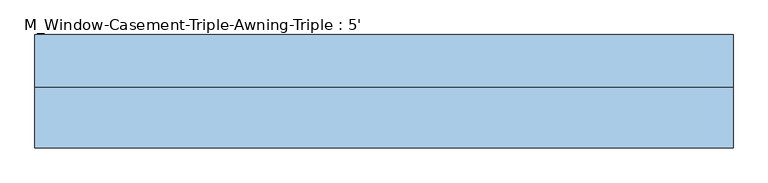
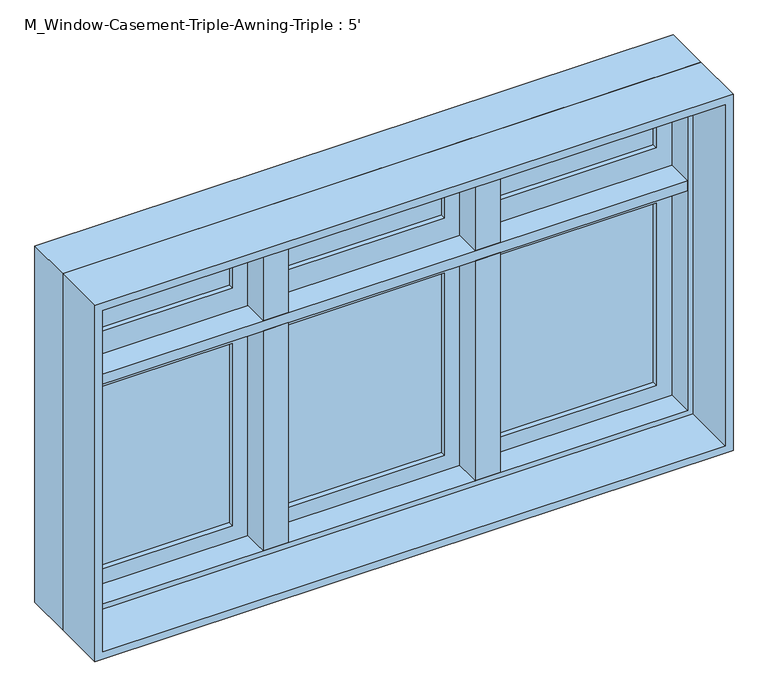
"""IFC4 building model written with IfcOpenShell, lengths in millimetres: window geometry, M_Window-Casement-Triple-Awning-Triple : 5'."""

from ifc_helpers import new_model, si_unit, frame, origin, place, context, project, spatial, polyline, outline, extrude, faceted_brep, source, transform, mapped, element, save


def m_window_casement_triple_awning_triple_5_96d5a87e(model_context):
    return source(origin(), model_context, "Body", "SolidModel", [
        faceted_brep([(730.25, 82.55, 1768.25), (730.25, 19.05, 1768.25), (-730.25, 19.05, 1768.25), (-730.25, 82.55, 1768.25), (749.3, 133.35, 1787.3), (749.3, 82.55, 1787.3), (-749.3, 82.55, 1787.3), (-749.3, 133.35, 1787.3), (762.0, 19.05, 1800.0), (762.0, 133.35, 1800.0), (-762.0, 133.35, 1800.0), (-762.0, 19.05, 1800.0), (-730.25, 19.05, 931.75), (-730.25, 82.55, 931.75), (-749.3, 82.55, 912.7), (-749.3, 133.35, 912.7), (-762.0, 133.35, 900.0), (-762.0, 19.05, 900.0), (730.25, 19.05, 931.75), (730.25, 82.55, 931.75), (749.3, 82.55, 912.7), (749.3, 133.35, 912.7), (762.0, 133.35, 900.0), (762.0, 19.05, 900.0)], [[[0, 1, 2, 3]], [[4, 5, 6, 7]], [[8, 9, 10, 11]], [[3, 2, 12, 13]], [[7, 6, 14, 15]], [[11, 10, 16, 17]], [[13, 12, 18, 19]], [[15, 14, 20, 21]], [[17, 16, 22, 23]], [[11, 17, 23, 8], [1, 18, 12, 2]], [[19, 18, 1, 0]], [[5, 20, 14, 6], [3, 13, 19, 0]], [[21, 20, 5, 4]], [[23, 22, 9, 8]], [[9, 22, 16, 10], [7, 15, 21, 4]]]),
        extrude(outline(polyline([(1800.0, -762.0), (900.0, -762.0), (900.0, 762.0), (1800.0, 762.0), (1800.0, -762.0)]), holes=[polyline([(1780.95, 742.95), (919.05, 742.95), (919.05, -742.95), (1780.95, -742.95), (1780.95, 742.95)])]), frame((0.0, -114.3, 0.0), z_axis=(0.0, 1.0, 0.0), x_axis=(0.0, 0.0, 1.0)), (0.0, 0.0, 1.0), 133.35),
        extrude(outline(polyline([(912.7, 749.3), (1487.3, 749.3), (1487.3, 262.4666667), (912.7, 262.4666667), (912.7, 749.3)]), holes=[polyline([(969.85, 319.6166667), (1430.15, 319.6166667), (1430.15, 692.15), (969.85, 692.15), (969.85, 319.6166667)])]), frame((0.0, 82.55, 0.0), z_axis=(0.0, 1.0, 0.0), x_axis=(0.0, 0.0, 1.0)), (0.0, 0.0, 1.0), 44.45),
        extrude(outline(polyline([(692.15, 114.3), (692.15, 107.95), (319.6166667, 107.95), (319.6166667, 114.3), (692.15, 114.3)])), frame((0.0, 0.0, 969.85), z_axis=(0.0, 0.0, 1.0), x_axis=(1.0, 0.0, 0.0)), (0.0, 0.0, 1.0), 460.3),
        extrude(outline(polyline([(319.6166667, 95.25), (319.6166667, 101.6), (692.15, 101.6), (692.15, 95.25), (319.6166667, 95.25)])), frame((0.0, 0.0, 969.85), z_axis=(0.0, 0.0, 1.0), x_axis=(1.0, 0.0, 0.0)), (0.0, 0.0, 1.0), 460.3),
        extrude(outline(polyline([(-319.6166667, 114.3), (-319.6166667, 107.95), (-692.15, 107.95), (-692.15, 114.3), (-319.6166667, 114.3)])), frame((0.0, 0.0, 969.85), z_axis=(0.0, 0.0, 1.0), x_axis=(1.0, 0.0, 0.0)), (0.0, 0.0, 1.0), 460.3),
        extrude(outline(polyline([(-692.15, 95.25), (-692.15, 101.6), (-319.6166667, 101.6), (-319.6166667, 95.25), (-692.15, 95.25)])), frame((0.0, 0.0, 969.85), z_axis=(0.0, 0.0, 1.0), x_axis=(1.0, 0.0, 0.0)), (0.0, 0.0, 1.0), 460.3),
        extrude(outline(polyline([(186.2666667, 114.3), (186.2666667, 107.95), (-186.2666667, 107.95), (-186.2666667, 114.3), (186.2666667, 114.3)])), frame((0.0, 0.0, 969.85), z_axis=(0.0, 0.0, 1.0), x_axis=(1.0, 0.0, 0.0)), (0.0, 0.0, 1.0), 460.3),
        extrude(outline(polyline([(-186.2666667, 95.25), (-186.2666667, 101.6), (186.2666667, 101.6), (186.2666667, 95.25), (-186.2666667, 95.25)])), frame((0.0, 0.0, 969.85), z_axis=(0.0, 0.0, 1.0), x_axis=(1.0, 0.0, 0.0)), (0.0, 0.0, 1.0), 460.3),
        faceted_brep([(-262.4666667, 82.55, 1487.3), (-282.9768005, 82.55, 1487.3), (-282.9768005, 19.05, 1487.3), (-222.9065328, 19.05, 1487.3), (-222.9065328, 82.55, 1487.3), (-243.4166667, 82.55, 1487.3), (-243.4166667, 133.35, 1487.3), (-262.4666667, 133.35, 1487.3), (-262.4666667, 133.35, 912.7), (-243.4166667, 133.35, 912.7), (-243.4166667, 95.25, 912.7), (-262.4666667, 95.25, 912.7), (-282.9768005, 82.55, 931.75), (-282.9768005, 19.05, 931.75), (-222.9065328, 19.05, 931.75), (-222.9065328, 82.55, 931.75), (-243.4166667, 82.55, 931.75), (-243.4166667, 95.25, 931.75), (-262.4666667, 95.25, 931.75), (-262.4666667, 82.55, 931.75)], [[[0, 1, 2, 3, 4, 5, 6, 7]], [[8, 9, 10, 11]], [[2, 1, 12, 13]], [[3, 2, 13, 14]], [[4, 3, 14, 15]], [[6, 5, 16, 17, 10, 9]], [[0, 7, 8, 11, 18, 19]], [[17, 18, 11, 10]], [[18, 17, 16, 15, 14, 13, 12, 19]], [[1, 0, 19, 12]], [[5, 4, 15, 16]], [[7, 6, 9, 8]]]),
        faceted_brep([(243.4166667, 82.55, 1487.3), (222.9065328, 82.55, 1487.3), (222.9065328, 19.05, 1487.3), (282.9768005, 19.05, 1487.3), (282.9768005, 82.55, 1487.3), (262.4666667, 82.55, 1487.3), (262.4666667, 133.35, 1487.3), (243.4166667, 133.35, 1487.3), (243.4166667, 133.35, 912.7), (262.4666667, 133.35, 912.7), (262.4666667, 95.25, 912.7), (243.4166667, 95.25, 912.7), (222.9065328, 82.55, 931.75), (222.9065328, 19.05, 931.75), (282.9768005, 19.05, 931.75), (282.9768005, 82.55, 931.75), (262.4666667, 82.55, 931.75), (262.4666667, 95.25, 931.75), (243.4166667, 95.25, 931.75), (243.4166667, 82.55, 931.75)], [[[0, 1, 2, 3, 4, 5, 6, 7]], [[8, 9, 10, 11]], [[2, 1, 12, 13]], [[3, 2, 13, 14]], [[4, 3, 14, 15]], [[6, 5, 16, 17, 10, 9]], [[0, 7, 8, 11, 18, 19]], [[17, 18, 11, 10]], [[18, 17, 16, 15, 14, 13, 12, 19]], [[1, 0, 19, 12]], [[5, 4, 15, 16]], [[7, 6, 9, 8]]]),
        extrude(outline(polyline([(-730.25, 19.05), (-730.25, 82.55), (-749.3, 82.55), (-749.3, 133.35), (749.3, 133.35), (749.3, 82.55), (730.25, 82.55), (730.25, 19.05), (-730.25, 19.05)])), frame((0.0, 0.0, 1487.3), z_axis=(0.0, 0.0, 1.0), x_axis=(1.0, 0.0, 0.0)), (0.0, 0.0, 1.0), 25.4),
        extrude(outline(polyline([(692.15, 114.3), (692.15, 107.95), (319.6166667, 107.95), (319.6166667, 114.3), (692.15, 114.3)])), frame((0.0, 0.0, 1569.85), z_axis=(0.0, 0.0, 1.0), x_axis=(1.0, 0.0, 0.0)), (0.0, 0.0, 1.0), 160.3),
        extrude(outline(polyline([(319.6166667, 101.6), (692.15, 101.6), (692.15, 95.25), (319.6166667, 95.25), (319.6166667, 101.6)])), frame((0.0, 0.0, 1569.85), z_axis=(0.0, 0.0, 1.0), x_axis=(1.0, 0.0, 0.0)), (0.0, 0.0, 1.0), 160.3),
        faceted_brep([(-243.4166667, 82.55, 1787.3), (-243.4166667, 133.35, 1787.3), (-262.4666667, 133.35, 1787.3), (-262.4666667, 82.55, 1787.3), (-262.4666667, 82.55, 1512.7), (-262.4666667, 133.35, 1512.7), (-243.4166667, 133.35, 1512.7), (-243.4166667, 82.55, 1512.7), (-222.9065328, 82.55, 1512.7), (-222.9065328, 19.05, 1512.7), (-282.9768005, 19.05, 1512.7), (-282.9768005, 82.55, 1512.7), (-282.9768005, 82.55, 1768.25), (-262.4666667, 82.55, 1768.25), (-282.9768005, 19.05, 1768.25), (-222.9065328, 19.05, 1768.25), (-222.9065328, 82.55, 1768.25), (-243.4166667, 82.55, 1768.25)], [[[0, 1, 2, 3]], [[4, 5, 6, 7, 8, 9, 10, 11]], [[4, 11, 12, 13]], [[11, 10, 14, 12]], [[10, 9, 15, 14]], [[9, 8, 16, 15]], [[8, 7, 17, 16]], [[1, 0, 17, 7, 6]], [[2, 1, 6, 5]], [[3, 2, 5, 4, 13]], [[17, 13, 12, 14, 15, 16]], [[13, 17, 0, 3]]]),
        faceted_brep([(262.4666667, 82.55, 1787.3), (262.4666667, 133.35, 1787.3), (243.4166667, 133.35, 1787.3), (243.4166667, 82.55, 1787.3), (243.4166667, 82.55, 1512.7), (243.4166667, 133.35, 1512.7), (262.4666667, 133.35, 1512.7), (262.4666667, 82.55, 1512.7), (282.9768005, 82.55, 1512.7), (282.9768005, 19.05, 1512.7), (222.9065328, 19.05, 1512.7), (222.9065328, 82.55, 1512.7), (222.9065328, 82.55, 1768.25), (243.4166667, 82.55, 1768.25), (222.9065328, 19.05, 1768.25), (282.9768005, 19.05, 1768.25), (282.9768005, 82.55, 1768.25), (262.4666667, 82.55, 1768.25)], [[[0, 1, 2, 3]], [[4, 5, 6, 7, 8, 9, 10, 11]], [[4, 11, 12, 13]], [[11, 10, 14, 12]], [[10, 9, 15, 14]], [[9, 8, 16, 15]], [[8, 7, 17, 16]], [[1, 0, 17, 7, 6]], [[2, 1, 6, 5]], [[3, 2, 5, 4, 13]], [[17, 13, 12, 14, 15, 16]], [[13, 17, 0, 3]]]),
        extrude(outline(polyline([(1512.7, 749.3), (1787.3, 749.3), (1787.3, 262.4666667), (1512.7, 262.4666667), (1512.7, 749.3)]), holes=[polyline([(1569.85, 319.6166667), (1730.15, 319.6166667), (1730.15, 692.15), (1569.85, 692.15), (1569.85, 319.6166667)])]), frame((0.0, 82.55, 0.0), z_axis=(0.0, 1.0, 0.0), x_axis=(0.0, 0.0, 1.0)), (0.0, 0.0, 1.0), 44.45),
        extrude(outline(polyline([(186.2666667, 114.3), (186.2666667, 107.95), (-186.2666667, 107.95), (-186.2666667, 114.3), (186.2666667, 114.3)])), frame((0.0, 0.0, 1569.85), z_axis=(0.0, 0.0, 1.0), x_axis=(1.0, 0.0, 0.0)), (0.0, 0.0, 1.0), 160.3),
        extrude(outline(polyline([(-186.2666667, 101.6), (186.2666667, 101.6), (186.2666667, 95.25), (-186.2666667, 95.25), (-186.2666667, 101.6)])), frame((0.0, 0.0, 1569.85), z_axis=(0.0, 0.0, 1.0), x_axis=(1.0, 0.0, 0.0)), (0.0, 0.0, 1.0), 160.3),
        extrude(outline(polyline([(-319.6166667, 114.3), (-319.6166667, 107.95), (-692.15, 107.95), (-692.15, 114.3), (-319.6166667, 114.3)])), frame((0.0, 0.0, 1569.85), z_axis=(0.0, 0.0, 1.0), x_axis=(1.0, 0.0, 0.0)), (0.0, 0.0, 1.0), 160.3),
        extrude(outline(polyline([(-692.15, 101.6), (-319.6166667, 101.6), (-319.6166667, 95.25), (-692.15, 95.25), (-692.15, 101.6)])), frame((0.0, 0.0, 1569.85), z_axis=(0.0, 0.0, 1.0), x_axis=(1.0, 0.0, 0.0)), (0.0, 0.0, 1.0), 160.3),
        extrude(outline(polyline([(1487.3, -243.4166667), (912.7, -243.4166667), (912.7, 243.4166667), (1487.3, 243.4166667), (1487.3, -243.4166667)]), holes=[polyline([(1430.15, 186.2666667), (969.85, 186.2666667), (969.85, -186.2666667), (1430.15, -186.2666667), (1430.15, 186.2666667)])]), frame((0.0, 82.55, 0.0), z_axis=(0.0, 1.0, 0.0), x_axis=(0.0, 0.0, 1.0)), (0.0, 0.0, 1.0), 44.45),
        extrude(outline(polyline([(1512.7, 243.4166667), (1787.3, 243.4166667), (1787.3, -243.4166667), (1512.7, -243.4166667), (1512.7, 243.4166667)]), holes=[polyline([(1569.85, -186.2666667), (1730.15, -186.2666667), (1730.15, 186.2666667), (1569.85, 186.2666667), (1569.85, -186.2666667)])]), frame((0.0, 82.55, 0.0), z_axis=(0.0, 1.0, 0.0), x_axis=(0.0, 0.0, 1.0)), (0.0, 0.0, 1.0), 44.45),
        extrude(outline(polyline([(1487.3, -749.3), (912.7, -749.3), (912.7, -262.4666667), (1487.3, -262.4666667), (1487.3, -749.3)]), holes=[polyline([(1430.15, -319.6166667), (969.85, -319.6166667), (969.85, -692.15), (1430.15, -692.15), (1430.15, -319.6166667)])]), frame((0.0, 82.55, 0.0), z_axis=(0.0, 1.0, 0.0), x_axis=(0.0, 0.0, 1.0)), (0.0, 0.0, 1.0), 44.45),
        extrude(outline(polyline([(1512.7, -262.4666667), (1787.3, -262.4666667), (1787.3, -749.3), (1512.7, -749.3), (1512.7, -262.4666667)]), holes=[polyline([(1569.85, -692.15), (1730.15, -692.15), (1730.15, -319.6166667), (1569.85, -319.6166667), (1569.85, -692.15)])]), frame((0.0, 82.55, 0.0), z_axis=(0.0, 1.0, 0.0), x_axis=(0.0, 0.0, 1.0)), (0.0, 0.0, 1.0), 44.45),
    ])


if __name__ == "__main__":
    model = new_model("IFC4")
    model_context = context("Model", 3, world=origin())
    ifc_project = project(units=[si_unit("LENGTHUNIT", "METRE", prefix="MILLI")], contexts=[model_context])
    site = spatial("IfcSite", under=ifc_project)
    building = spatial("IfcBuilding", under=site)
    placement = place(None, origin())
    m_window_casement_triple_awning_triple_5_shape = m_window_casement_triple_awning_triple_5_96d5a87e(model_context)
    element("IfcWindow", 1, ObjectType="M_Window-Casement-Triple-Awning-Triple : 5'", at=placement, inside=building, context=model_context, shape_type="MappedRepresentation", body=[
        mapped(m_window_casement_triple_awning_triple_5_shape, transform((0.0, 0.0, 0.0), x_axis=(1.0, 0.0, 0.0), y_axis=(0.0, 1.0, 0.0), z_axis=(0.0, 0.0, 1.0))),
    ])
    save(model, "model.ifc")

# Revit data of these elements
# Type "M_Window-Casement-Triple-Awning-Triple : 5'"
#   Type Mark = "19"
#   Fire Rating = "0.5h"
#   Assembly Code = "B2020100"
#   Analytic Construction = "Double glazing - domestic"
#   Window Inset [instance default] = 0' - 0"
#   Wall Thickness [instance default] = 0' - 5.90551"
#   One Third Width = 1' - 8"
#   Visual Light Transmittance = 0.81
#   Transom Height = 0' - 11.81102"
#   Thermal Resistance (R) = 1.8146 (h·ft²·°F)/BTU
#   Solar Heat Gain Coefficient = 0.76
#   Sash Width = 1' - 7.16667"
#   Rough Width = 5' - 0.59055"
#   Rough Height = 3' - 0.02362"
#   Open Window Height = 1' - 11.62205"
#   Frame Extension [instance default] = 0' - 0 1/4"
#   Interior Wall Closure [instance default] = 0' - 2.15551"
#   Height = 2' - 11.43307"
#   Heat Transfer Coefficient (U) = 0.5511 BTU/(h·ft²·°F)
#   Exterior Wall Closure [instance default] = 0' - 1 1/4"
#   Extension Jamb [instance default] = 0' - 2.15551"
#   Default Sill Height = 2' - 11.43307"
#   Width = 5' - 0"
#   Top Side Muntin Visibility = yes
#   Top Middle Muntin Visibility = yes
#   Bottom Side Muntin Visibility = yes
#   Bottom Middle Muntin Visibility = yes
#   Interior Trim Visibility [instance default] = yes
#   Exterior Trim Visibility [instance default] = yes
#   Extension Jamb Visibility [instance default] = yes
#   Muntin Pattern = M_Muntin Pattern_2x2 : M_Muntin Pattern_2x2
#   Interior Trim Material = Wood - Stained
#   Interior Trim = M_Trim-Window-Interior-Flat : Picture Frame
#   Interior Frame Material = Wood - Stained
#   Glass Panel Material = Glass
#   Exterior Trim Material = Clad - White
#   Exterior Trim = M_Trim-Window-Exterior-Flat : with Sill
#   Exterior Frame Material = Clad - White
#   Wall Closure = (empty or 0)
# Element 1 (IfcWindow, "M_Window-Casement-Triple-Awning-Triple : 5'")
#   Wall Thickness = 0' - 9"
#   Extension Jamb = 0' - 5 1/4"
#   Materials on its faces: "Wood - Stained", "Glass", "Clad - White"
# Materials
#   "Wood - Stained": class "Wood", colour RGB 224 178 126, transparency 0, Cost = 0
#   "Glass": class "Glass", colour RGB 0 128 192, transparency 0.75, Description = "Soda Lime Glass", Cost = 0
#   "Clad - White": class "Wood", colour RGB 242 242 238, transparency 0, Cost = 0
